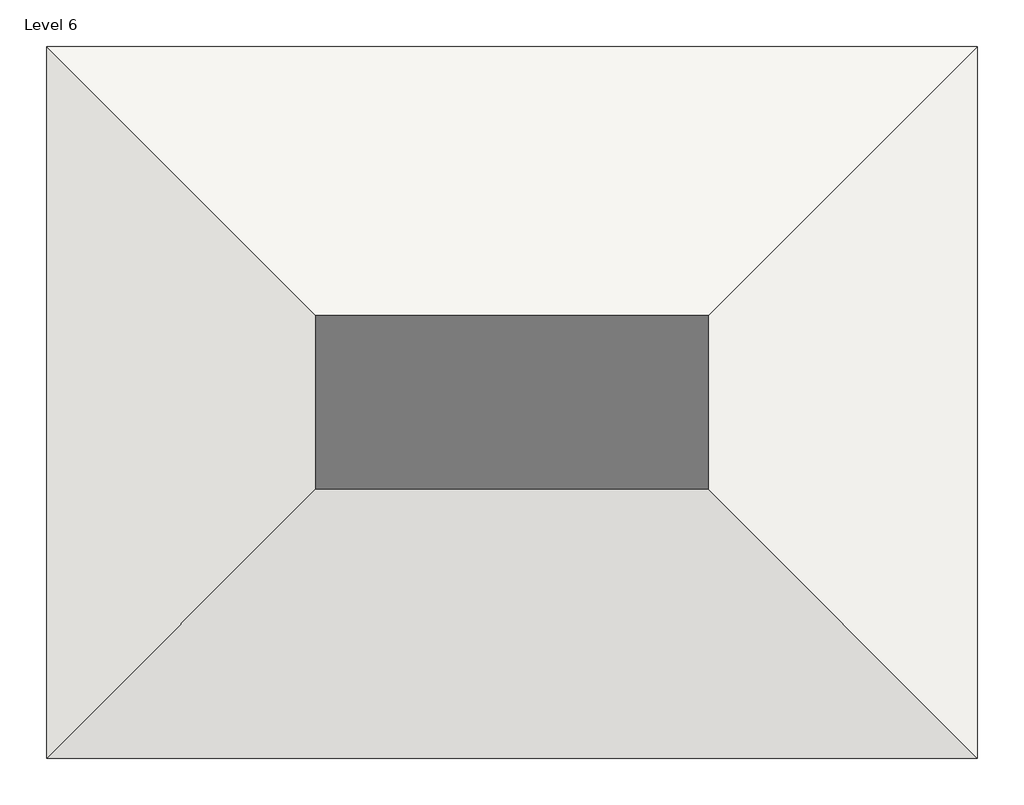
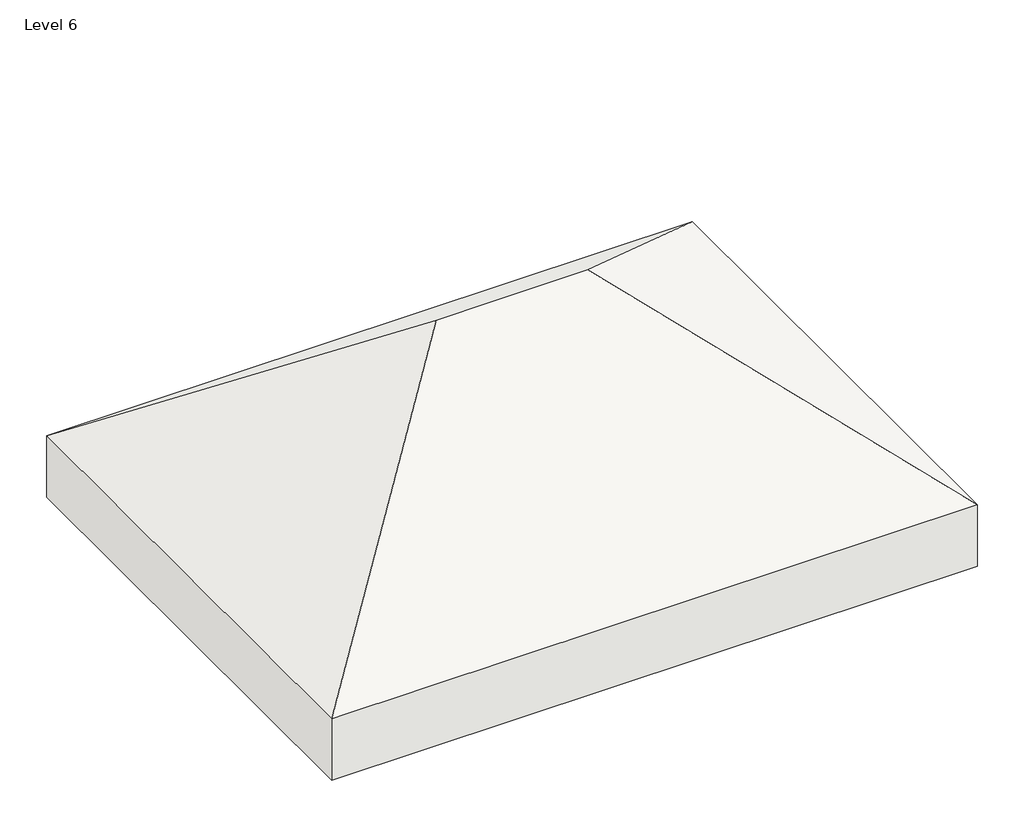
# One storey: 1 roof.
"""IFC4 building model written with IfcOpenShell, lengths in millimetres."""

from ifc_helpers import new_model, si_unit, origin, place, context, project, spatial, faceted_brep, element, save

model = new_model("IFC4")

# Units and contexts
model_context = context("Model", 3, world=origin())
ifc_project = project(units=[si_unit("LENGTHUNIT", "METRE", prefix="MILLI")], contexts=[model_context])

# Site, building, storey
site = spatial("IfcSite", under=ifc_project)
building = spatial("IfcBuilding", under=site)
storey = spatial("IfcBuildingStorey", under=building, Name="Level 6", Elevation=8534.4)

# Roof
placement = place(None, origin())
element("IfcRoof", 1, ObjectType="ROOFING 1'", at=placement, inside=storey, context=model_context, shape_type="Brep", body=[
    faceted_brep([(-8328.1357439, 2761.0172538, 9620.25), (-9775.9357439, 4208.8172538, 8534.4), (-5989.7482439, 4208.8172538, 8534.4), (-7437.5482439, 2761.0172538, 9620.25), (-5989.7482439, 1313.2172538, 8534.4), (-9775.9357439, 1313.2172538, 8534.4), (-9775.9357439, 4208.8172538, 8915.4), (-8328.1357439, 2761.0172538, 10001.25), (-7437.5482439, 2761.0172538, 10001.25), (-5989.7482439, 4208.8172538, 8915.4), (-5989.7482439, 1313.2172538, 8915.4), (-9775.9357439, 1313.2172538, 8915.4)], [[[0, 1, 2, 3]], [[4, 3, 2]], [[5, 0, 3, 4]], [[1, 0, 5]], [[6, 7, 8, 9]], [[10, 9, 8]], [[11, 10, 8, 7]], [[6, 11, 7]], [[5, 11, 6, 1]], [[4, 10, 11, 5]], [[2, 9, 10, 4]], [[1, 6, 9, 2]]]),
])

save(model, "model.ifc")

# Revit data of these elements
# Type "ROOFING 1'"
#   Assembly Code = "B1020"
#   Layers, outside or top first: 1' - 0" "ROOFING 1'" (function 1)
# Element 1 (IfcRoof, "ROOFING 1'")
#   built-in parameter 1001705 = 32.8125 (stored number, unit not read)
#   built-in parameter 1001710 = 33615
#   Phase Created = New Construction
#   Materials on its faces: "ROOFING 1'"
# Materials
#   "ROOFING 1'": class "Generic", colour RGB 120 120 120, transparency 0, Cost = 0
